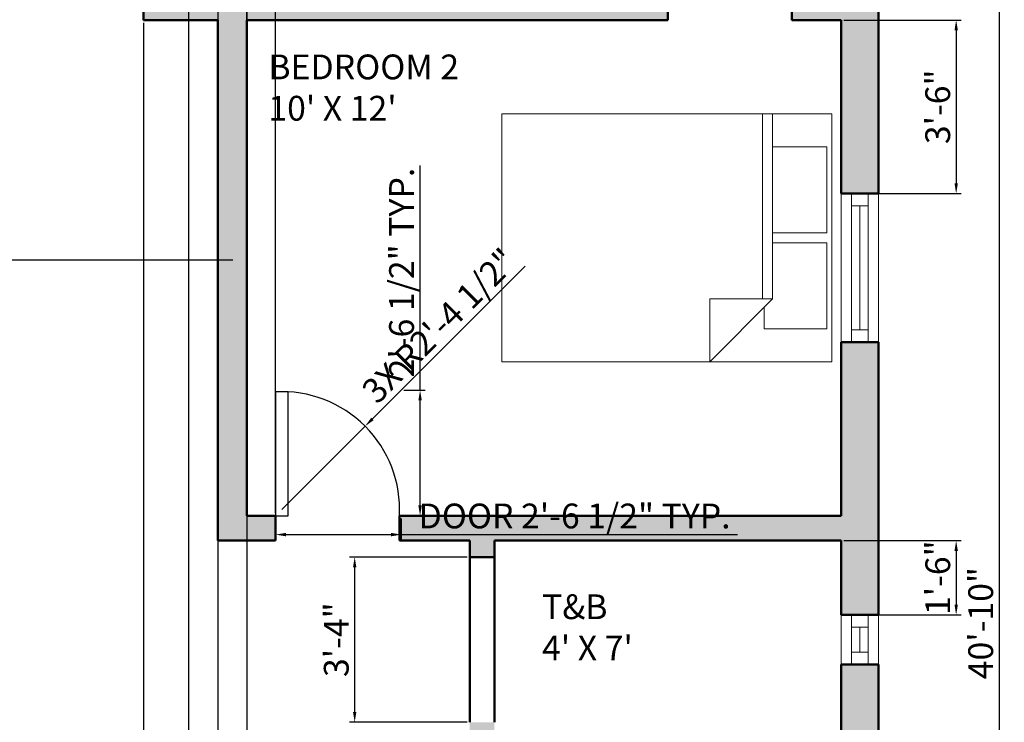
# Model space of a CAD drawing. Units: inches. Extents: x 2247 to 2697, y 1573 to 2133.
# Tile 3 of 4: x 2409 to 2648, y 1823 to 1993. Entities that reach past the tile are written whole.
import ezdxf

# ---------------------------------------------------------------- set-up
doc = ezdxf.new("R2010")
doc.units = ezdxf.units.IN
for name, color, linetype, lineweight in [('A-ANNO-DIMS', 2, 'Continuous', 18), ('A-AREA-IDEN', 7, 'Continuous', 25), ('A-DOOR', 4, 'Continuous', 25), ('A-FURN', 8, 'Continuous', 18), ('A-GLAZ', 4, 'Continuous', 18), ('A-WALL', 7, 'Continuous', 50)]:
    doc.layers.add(name, color=color, linetype=linetype, lineweight=lineweight)
doc.layers.add('A-WALL-PATT', color=67, linetype='Continuous', lineweight=13, true_color=0x727430)
doc.styles.get("Standard").update_dxf_attribs({"font": 'arial.ttf'})
doc.dimstyles.new('ISO-25', dxfattribs={"dimtxt": 6, "dimasz": 2.5, "dimexe": 1.25, "dimexo": 0.625, "dimtad": 1, "dimlunit": 3, "dimtxsty": 'Standard', "dimcen": 2.5, "dimadec": 0, "dimazin": 0, "dimtfac": 1, "dimtmove": 0, "dimatfit": 3, "dimfxl": 1, "dimarcsym": 0})

# ---------------------------------------------------------------- blocks, each defined once
blk = doc.blocks.new('*D2')
at = {"layer": 'A-ANNO-DIMS', "color": 0, "lineweight": -2, "transparency": 16777216}
for p, q in [((2617.72, 2092.36), (2647.6, 2092.36)), ((2646.35, 2089.86), (2646.35, 1604.86)), ((2617.72, 1602.36), (2647.6, 1602.36))]:
    blk.add_line(p, q, dxfattribs=at)
at = {"layer": 'A-ANNO-DIMS', "color": 0, "transparency": 16777216}
for points in [[(2645.94, 2089.86), (2646.77, 2089.86), (2646.35, 2092.36)], [(2645.94, 1604.86), (2646.77, 1604.86), (2646.35, 1602.36)]]:
    blk.add_solid(points, dxfattribs=at)
at = {"layer": 'Defpoints', "color": 0, "transparency": 16777216}
for p in [(2617.09, 2092.36), (2617.09, 1602.36), (2646.35, 1602.36)]:
    blk.add_point(p, dxfattribs=at)
at = {"layer": 'A-ANNO-DIMS', "color": 0, "transparency": 16777216, "insert": (2642.66, 1847.36), "char_height": 6, "attachment_point": 5, "rotation": 90}
blk.add_mtext('40\'-10"', dxfattribs=at)
blk = doc.blocks.new('Bed - Queen')
for p, q in [((0, -80.00003), (0, 0)), ((0, 0), (59.99999, 0)), ((59.99999, 0), (59.99999, -80.00003)), ((7.99999, -1.2), (28.79998, -1.2)), ((7.99999, -14.4), (7.99999, -1.2)), ((28.79998, -1.2), (28.79998, -14.4)), ((31.19999, -1.2), (51.99999, -1.2)), ((31.19999, -14.4), (31.19999, -1.2)), ((51.99999, -1.2), (51.99999, -16.4)), ((0, -14.4), (44.8, -14.4)), ((59.99999, -29.6), (44.8, -14.4)), ((44.8, -14.4), (44.8, -29.6)), ((51.99999, -16.4), (46.79936, -16.4)), ((44.8, -16.8), (0, -16.8)), ((44.8, -29.6), (59.99999, -29.6)), ((59.99999, -80.00003), (0, -80.00003))]:
    blk.add_line(p, q)
blk = doc.blocks.new('DOOR-SWING-30IN')
blk.add_lwpolyline([(0, 0), (3, 0), (3, 30), (0, 30)], close=True)
blk.add_arc((1.5, 1.5), 28.54, 356.9872, 93.0128)
blk = doc.blocks.new('WIN-36IN')
for p, q in [((0, 9), (36, 9)), ((0, 6.5), (36, 6.5)), ((3, 2.5), (3, 6.5)), ((33, 2.5), (33, 6.5)), ((0, 2.5), (36, 2.5)), ((3, 4.5), (33, 4.5)), ((0, 0), (36, 0))]:
    blk.add_line(p, q)
blk = doc.blocks.new('WIN-SASH-12IN')
for p, q in [((0, 0), (0, 12)), ((4, 0), (4, 12)), ((0, 9), (4, 9)), ((2, 3), (2, 9)), ((0, 3), (4, 3))]:
    blk.add_line(p, q)
blk = doc.blocks.new('*D11')
at = {"layer": 'A-ANNO-DIMS', "color": 0, "lineweight": -2, "transparency": 16777216}
for p, q in [((2471.09, 1872.73), (2471.09, 1867.55)), ((2501.52, 1872.73), (2501.52, 1867.55)), ((2473.59, 1868.8), (2499.02, 1868.8)), ((2501.52, 1868.8), (2583, 1868.8))]:
    blk.add_line(p, q, dxfattribs=at)
at = {"layer": 'A-ANNO-DIMS', "color": 0, "transparency": 16777216}
for points in [[(2473.59, 1869.21), (2473.59, 1868.38), (2471.09, 1868.8)], [(2499.02, 1869.21), (2499.02, 1868.38), (2501.52, 1868.8)]]:
    blk.add_solid(points, dxfattribs=at)
at = {"layer": 'Defpoints', "color": 0, "transparency": 16777216}
for p in [(2471.09, 1873.36), (2501.52, 1873.36), (2501.52, 1868.8)]:
    blk.add_point(p, dxfattribs=at)
at = {"layer": 'A-ANNO-DIMS', "color": 0, "transparency": 16777216, "insert": (2543.51, 1872.53), "char_height": 6, "attachment_point": 5}
blk.add_mtext('DOOR 2\'-6 1/2" TYP.', dxfattribs=at)
blk = doc.blocks.new('*D12')
at = {"layer": 'A-ANNO-DIMS', "color": 0, "lineweight": -2, "transparency": 16777216}
for p, q in [((2506.08, 1903.78), (2506.08, 1958.19)), ((2502.14, 1903.78), (2507.33, 1903.78)), ((2506.08, 1875.86), (2506.08, 1901.28)), ((2502.14, 1873.36), (2507.33, 1873.36))]:
    blk.add_line(p, q, dxfattribs=at)
at = {"layer": 'A-ANNO-DIMS', "color": 0, "transparency": 16777216}
for points in [[(2505.67, 1901.28), (2506.5, 1901.28), (2506.08, 1903.78)], [(2505.67, 1875.86), (2506.5, 1875.86), (2506.08, 1873.36)]]:
    blk.add_solid(points, dxfattribs=at)
at = {"layer": 'Defpoints', "color": 0, "transparency": 16777216}
for p in [(2501.52, 1903.78), (2506.08, 1903.78), (2501.52, 1873.36)]:
    blk.add_point(p, dxfattribs=at)
at = {"layer": 'A-ANNO-DIMS', "color": 0, "transparency": 16777216, "insert": (2502.36, 1932.24), "char_height": 6, "attachment_point": 5, "rotation": 90}
blk.add_mtext('2\'-6 1/2" TYP.', dxfattribs=at)
blk = doc.blocks.new('*D26')
at = {"layer": 'A-ANNO-DIMS', "color": 0, "lineweight": -2, "transparency": 16777216}
for p, q in [((2457.09, 2052.73), (2457.09, 1573.26)), ((2464.09, 2052.73), (2464.09, 1573.26)), ((2459.59, 1574.51), (2461.59, 1574.51)), ((2464.09, 1574.51), (2483.79, 1574.51))]:
    blk.add_line(p, q, dxfattribs=at)
at = {"layer": 'A-ANNO-DIMS', "color": 0, "transparency": 16777216}
for points in [[(2459.59, 1574.93), (2459.59, 1574.09), (2457.09, 1574.51)], [(2461.59, 1574.93), (2461.59, 1574.09), (2464.09, 1574.51)]]:
    blk.add_solid(points, dxfattribs=at)
at = {"layer": 'Defpoints', "color": 0, "transparency": 16777216}
for p in [(2457.09, 2053.36), (2464.09, 2053.36), (2464.09, 1574.51)]:
    blk.add_point(p, dxfattribs=at)
at = {"layer": 'A-ANNO-DIMS', "color": 0, "transparency": 16777216, "insert": (2475.19, 1578.2), "char_height": 6, "attachment_point": 5}
blk.add_mtext('0\'-7"', dxfattribs=at)
blk = doc.blocks.new('*D28')
at = {"layer": 'A-ANNO-DIMS', "color": 0, "lineweight": -2, "transparency": 16777216}
for p, q in [((2608.72, 1993.36), (2637.19, 1993.36)), ((2635.94, 1990.86), (2635.94, 1953.86)), ((2608.72, 1951.36), (2637.19, 1951.36))]:
    blk.add_line(p, q, dxfattribs=at)
at = {"layer": 'A-ANNO-DIMS', "color": 0, "transparency": 16777216}
for points in [[(2635.53, 1990.86), (2636.36, 1990.86), (2635.94, 1993.36)], [(2635.53, 1953.86), (2636.36, 1953.86), (2635.94, 1951.36)]]:
    blk.add_solid(points, dxfattribs=at)
at = {"layer": 'Defpoints', "color": 0, "transparency": 16777216}
for p in [(2608.09, 1993.36), (2608.09, 1951.36), (2635.94, 1951.36)]:
    blk.add_point(p, dxfattribs=at)
at = {"layer": 'A-ANNO-DIMS', "color": 0, "transparency": 16777216, "insert": (2632.25, 1972.36), "char_height": 6, "attachment_point": 5, "rotation": 90}
blk.add_mtext('3\'-6"', dxfattribs=at)
blk = doc.blocks.new('*D29')
at = {"layer": 'A-ANNO-DIMS', "color": 0, "lineweight": -2, "transparency": 16777216}
for p, q in [((2608.72, 1867.36), (2637.19, 1867.36)), ((2635.94, 1864.86), (2635.94, 1851.86)), ((2608.72, 1849.36), (2637.19, 1849.36))]:
    blk.add_line(p, q, dxfattribs=at)
at = {"layer": 'A-ANNO-DIMS', "color": 0, "transparency": 16777216}
for points in [[(2635.53, 1864.86), (2636.36, 1864.86), (2635.94, 1867.36)], [(2635.53, 1851.86), (2636.36, 1851.86), (2635.94, 1849.36)]]:
    blk.add_solid(points, dxfattribs=at)
at = {"layer": 'Defpoints', "color": 0, "transparency": 16777216}
for p in [(2608.09, 1867.36), (2608.09, 1849.36), (2635.94, 1849.36)]:
    blk.add_point(p, dxfattribs=at)
at = {"layer": 'A-ANNO-DIMS', "color": 0, "transparency": 16777216, "insert": (2632.26, 1858.36), "char_height": 6, "attachment_point": 5, "rotation": 90}
blk.add_mtext('1\'-6"', dxfattribs=at)
blk = doc.blocks.new('*D38')
at = {"layer": 'A-ANNO-DIMS', "color": 0, "lineweight": -2, "transparency": 16777216}
for p, q in [((2390.09, 1693.98), (2390.09, 2121.46)), ((2450.09, 1693.98), (2450.09, 2121.46)), ((2392.59, 2120.21), (2447.59, 2120.21))]:
    blk.add_line(p, q, dxfattribs=at)
at = {"layer": 'A-ANNO-DIMS', "color": 0, "transparency": 16777216}
for points in [[(2392.59, 2120.63), (2392.59, 2119.79), (2390.09, 2120.21)], [(2447.59, 2120.63), (2447.59, 2119.79), (2450.09, 2120.21)]]:
    blk.add_solid(points, dxfattribs=at)
at = {"layer": 'Defpoints', "color": 0, "transparency": 16777216}
for p in [(2450.09, 2120.21), (2390.09, 1693.36), (2450.09, 1693.36)]:
    blk.add_point(p, dxfattribs=at)
at = {"layer": 'A-ANNO-DIMS', "color": 0, "transparency": 16777216, "insert": (2420.09, 2123.9), "char_height": 6, "attachment_point": 5}
blk.add_mtext('5\'-0"', dxfattribs=at)
blk = doc.blocks.new('*D40')
at = {"layer": 'A-ANNO-DIMS', "color": 0, "lineweight": -2, "transparency": 16777216}
for p, q in [((2391.09, 1992.73), (2391.09, 1573.26)), ((2439.09, 1992.73), (2439.09, 1573.26)), ((2393.59, 1574.51), (2436.59, 1574.51))]:
    blk.add_line(p, q, dxfattribs=at)
at = {"layer": 'A-ANNO-DIMS', "color": 0, "transparency": 16777216}
for points in [[(2393.59, 1574.93), (2393.59, 1574.09), (2391.09, 1574.51)], [(2436.59, 1574.93), (2436.59, 1574.09), (2439.09, 1574.51)]]:
    blk.add_solid(points, dxfattribs=at)
at = {"layer": 'Defpoints', "color": 0, "transparency": 16777216}
for p in [(2391.09, 1993.36), (2439.09, 1993.36), (2439.09, 1574.51)]:
    blk.add_point(p, dxfattribs=at)
at = {"layer": 'A-ANNO-DIMS', "color": 0, "transparency": 16777216, "insert": (2415.09, 1578.2), "char_height": 6, "attachment_point": 5}
blk.add_mtext('4\'-0"', dxfattribs=at)
blk = doc.blocks.new('*D42')
at = {"layer": 'A-ANNO-DIMS', "color": 0, "lineweight": -2, "transparency": 16777216}
for p, q in [((2464.09, 1873.98), (2464.09, 2121.46)), ((2471.09, 1873.98), (2471.09, 2121.46)), ((2466.59, 2120.21), (2468.59, 2120.21)), ((2471.09, 2120.21), (2490.79, 2120.21))]:
    blk.add_line(p, q, dxfattribs=at)
at = {"layer": 'A-ANNO-DIMS', "color": 0, "transparency": 16777216}
for points in [[(2466.59, 2120.63), (2466.59, 2119.79), (2464.09, 2120.21)], [(2468.59, 2120.63), (2468.59, 2119.79), (2471.09, 2120.21)]]:
    blk.add_solid(points, dxfattribs=at)
at = {"layer": 'Defpoints', "color": 0, "transparency": 16777216}
for p in [(2471.09, 2120.21), (2464.09, 1873.36), (2471.09, 1873.36)]:
    blk.add_point(p, dxfattribs=at)
at = {"layer": 'A-ANNO-DIMS', "color": 0, "transparency": 16777216, "insert": (2482.19, 2123.9), "char_height": 6, "attachment_point": 5}
blk.add_mtext('0\'-7"', dxfattribs=at)
blk = doc.blocks.new('*D44')
at = {"layer": 'A-ANNO-DIMS', "color": 0, "lineweight": -2, "transparency": 16777216}
for p, q in [((2517.47, 1863.36), (2488.99, 1863.36)), ((2490.24, 1825.86), (2490.24, 1860.86)), ((2517.47, 1823.36), (2488.99, 1823.36))]:
    blk.add_line(p, q, dxfattribs=at)
at = {"layer": 'A-ANNO-DIMS', "color": 0, "transparency": 16777216}
for points in [[(2489.83, 1860.86), (2490.66, 1860.86), (2490.24, 1863.36)], [(2489.83, 1825.86), (2490.66, 1825.86), (2490.24, 1823.36)]]:
    blk.add_solid(points, dxfattribs=at)
at = {"layer": 'Defpoints', "color": 0, "transparency": 16777216}
for p in [(2490.24, 1863.36), (2518.09, 1863.36), (2518.09, 1823.36)]:
    blk.add_point(p, dxfattribs=at)
at = {"layer": 'A-ANNO-DIMS', "color": 0, "transparency": 16777216, "insert": (2486.55, 1843.36), "char_height": 6, "attachment_point": 5, "rotation": 90}
blk.add_mtext('3\'-4"', dxfattribs=at)
blk = doc.blocks.new('*D49')
at = {"layer": 'A-ANNO-DIMS', "color": 0, "lineweight": -2, "transparency": 16777216}
for p, q in [((2252.99, 1935.2), (2337.01, 1935.2)), ((2460.71, 1935.2), (2339.51, 1935.2))]:
    blk.add_line(p, q, dxfattribs=at)
at = {"layer": 'A-ANNO-DIMS', "color": 0, "transparency": 16777216}
blk.add_solid([(2337.01, 1935.62), (2337.01, 1934.79), (2339.51, 1935.2)], dxfattribs=at)
at = {"layer": 'Defpoints', "color": 0, "transparency": 16777216}
for p in [(2339.51, 1935.2), (2460.71, 1935.2)]:
    blk.add_point(p, dxfattribs=at)
at = {"layer": 'A-ANNO-DIMS', "color": 0, "transparency": 16777216, "insert": (2266.79, 1938.89), "char_height": 6, "attachment_point": 5}
blk.add_mtext('R10\'-1"', dxfattribs=at)
blk = doc.blocks.new('*D50')
at = {"layer": 'A-ANNO-DIMS', "color": 0, "lineweight": -2, "transparency": 16777216}
for p, q in [((2246.5, 1935.2), (2331.01, 1935.2)), ((2447.76, 1935.2), (2333.51, 1935.2))]:
    blk.add_line(p, q, dxfattribs=at)
at = {"layer": 'A-ANNO-DIMS', "color": 0, "transparency": 16777216}
blk.add_solid([(2331.01, 1935.62), (2331.01, 1934.79), (2333.51, 1935.2)], dxfattribs=at)
at = {"layer": 'Defpoints', "color": 0, "transparency": 16777216}
for p in [(2333.51, 1935.2), (2447.76, 1935.2)]:
    blk.add_point(p, dxfattribs=at)
at = {"layer": 'A-ANNO-DIMS', "color": 0, "transparency": 16777216, "insert": (2264.96, 1938.93), "char_height": 6, "attachment_point": 5}
blk.add_mtext('R9\'-6 1/2"', dxfattribs=at)
blk = doc.blocks.new('*D51')
at = {"layer": 'A-ANNO-DIMS', "color": 0, "lineweight": -2, "transparency": 16777216}
for p, q in [((2531.53, 1933.8), (2494.54, 1896.81)), ((2472.59, 1874.86), (2492.77, 1895.04))]:
    blk.add_line(p, q, dxfattribs=at)
at = {"layer": 'A-ANNO-DIMS', "color": 0, "transparency": 16777216}
blk.add_solid([(2494.25, 1897.1), (2494.84, 1896.51), (2492.77, 1895.04)], dxfattribs=at)
at = {"layer": 'Defpoints', "color": 0, "transparency": 16777216}
for p in [(2492.77, 1895.04), (2472.59, 1874.86)]:
    blk.add_point(p, dxfattribs=at)
at = {"layer": 'A-ANNO-DIMS', "color": 0, "transparency": 16777216, "insert": (2511.28, 1918.82), "char_height": 6, "attachment_point": 5, "rotation": 44.9996}
blk.add_mtext('3X R2\'-4 1/2"', dxfattribs=at)

msp = doc.modelspace()

# ---------------------------------------------------------------- hatches: boundary and pattern name
at = {"layer": 'A-WALL-PATT'}
h = msp.add_hatch(color=256, dxfattribs=at)
h.dxf.hatch_style = 1
h.paths.add_polyline_path([(2566.094, 1999.36), (2559.094, 1999.36), (2559.094, 2083.36), (2607.094, 2083.36), (2607.094, 2047.36), (2617.094, 2047.36), (2617.094, 2092.36), (2526.594, 2092.36), (2526.594, 2083.36), (2553.094, 2083.36), (2553.094, 1999.36), (2464.094, 1999.36), (2439.094, 1999.36), (2439.094, 1993.36), (2457.094, 1993.36), (2457.094, 1867.36), (2471.094, 1867.36), (2471.094, 1873.36), (2464.094, 1873.36), (2464.094, 1993.36), (2566.094, 1993.36)])
h = msp.add_hatch(color=256, dxfattribs=at)
h.dxf.hatch_style = 1
h.paths.add_polyline_path([(2617.094, 2035.36), (2607.094, 2035.36), (2607.094, 1999.36), (2596.094, 1999.36), (2596.094, 1993.36), (2608.094, 1993.36), (2608.094, 1951.36), (2617.094, 1951.36)])
h = msp.add_hatch(color=256, dxfattribs=at)
h.dxf.hatch_style = 1
h.paths.add_polyline_path([(2617.094, 1915.36), (2608.094, 1915.36), (2608.094, 1873.36), (2501.094, 1873.36), (2501.094, 1867.36), (2518.094, 1867.36), (2518.094, 1863.36), (2524.094, 1863.36), (2524.094, 1867.36), (2608.094, 1867.36), (2608.094, 1849.36), (2617.094, 1849.36)])
h = msp.add_hatch(color=256, dxfattribs=at)
h.dxf.hatch_style = 1
h.paths.add_polyline_path([(2617.094, 1837.36), (2608.094, 1837.36), (2608.094, 1819.36), (2524.094, 1819.36), (2524.094, 1823.36), (2518.094, 1823.36), (2518.094, 1819.36), (2501.094, 1819.36), (2501.094, 1813.36), (2608.094, 1813.36), (2608.094, 1771.36), (2617.094, 1771.36)])

# ---------------------------------------------------------------- linework, layer by layer
at = {"layer": 'A-GLAZ'}
for p, q in [((2608.094, 1849.36), (2608.094, 1837.36)), ((2617.094, 1837.36), (2617.094, 1849.36))]:
    msp.add_line(p, q, dxfattribs=at)
at = {"layer": 'A-WALL'}
for p, q in [((2439.094, 1993.36), (2439.094, 1999.36)), ((2566.094, 1999.36), (2566.094, 1993.36)), ((2596.094, 1999.36), (2596.094, 1993.36)), ((2439.094, 1993.36), (2457.094, 1993.36)), ((2457.094, 1867.36), (2457.094, 1993.36)), ((2464.094, 1993.36), (2464.094, 1873.36)), ((2464.094, 1993.36), (2566.094, 1993.36)), ((2596.094, 1993.36), (2608.094, 1993.36)), ((2608.094, 1993.36), (2608.094, 1951.36)), ((2608.094, 1951.36), (2617.094, 1951.36)), ((2608.094, 1915.36), (2617.094, 1915.36)), ((2608.094, 1915.36), (2608.094, 1873.36)), ((2464.094, 1873.36), (2471.094, 1873.36)), ((2471.094, 1873.36), (2471.094, 1867.36)), ((2501.094, 1873.36), (2501.094, 1867.36)), ((2501.094, 1873.36), (2608.094, 1873.36)), ((2457.094, 1867.36), (2471.094, 1867.36)), ((2501.094, 1867.36), (2518.094, 1867.36)), ((2518.094, 1867.36), (2518.094, 1863.36)), ((2524.094, 1867.36), (2524.094, 1863.36)), ((2524.094, 1867.36), (2608.094, 1867.36)), ((2608.094, 1867.36), (2608.094, 1849.36)), ((2518.094, 1863.36), (2524.094, 1863.36)), ((2518.094, 1823.36), (2518.094, 1863.36)), ((2524.094, 1823.36), (2524.094, 1863.36)), ((2608.094, 1849.36), (2617.094, 1849.36)), ((2608.094, 1837.36), (2617.094, 1837.36)), ((2608.094, 1837.36), (2608.094, 1819.36))]:
    msp.add_line(p, q, dxfattribs=at)
for points in [[(2617.094, 2035.36), (2617.094, 1951.36)], [(2617.094, 1915.36), (2617.094, 1849.36)], [(2617.094, 1837.36), (2617.094, 1771.36)]]:
    msp.add_lwpolyline(points, dxfattribs=at)

# ---------------------------------------------------------------- block references
at = {"layer": 'A-DOOR'}
msp.add_blockref('DOOR-SWING-30IN', (2471.094, 1873.36), dxfattribs=at)
at = {"layer": 'A-FURN', "rotation": 270}
msp.add_blockref('Bed - Queen', (2605.851, 1970.648), dxfattribs=at)
at = {"layer": 'A-GLAZ'}
for name, p, rotation in [('WIN-36IN', (2608.095, 1951.36), 270.0000000000049), ('WIN-SASH-12IN', (2614.595, 1849.359), 180)]:
    msp.add_blockref(name, p, dxfattribs=dict(at, rotation=rotation))

# ---------------------------------------------------------------- texts
at = {"layer": 'A-AREA-IDEN', "char_height": 6, "attachment_point": 1}
for s, width, insert in [("{\\fArial|b1|i0|c0|p34;BEDROOM 2 \\P10' X 12'}", 104.07009, (2469.331, 1985.018)), ("{\\fArial|b1|i0|c0|p34;T&B \\P4' X 7'}", 43.11494, (2535.625, 1854.335))]:
    msp.add_mtext_dynamic_manual_height_columns(s, width=width, gutter_width=12.5, heights=[0], dxfattribs=dict(at, insert=insert))

# ---------------------------------------------------------------- dimensions: what is measured, and where the dimension line sits
at = {"layer": 'A-ANNO-DIMS'}
for base, p1, p2, picture, middle in [((2450.094, 2120.21), (2390.094, 1693.36), (2450.094, 1693.36), '*D38', (2420.094, 2123.898)), ((2471.094, 2120.21), (2464.094, 1873.36), (2471.094, 1873.36), '*D42', (2482.194, 2123.898)), ((2464.094, 1574.51), (2457.094, 2053.36), (2464.094, 2053.36), '*D26', (2475.194, 1578.198)), ((2439.094, 1574.51), (2391.094, 1993.36), (2439.094, 1993.36), '*D40', (2415.094, 1578.198))]:
    dim = msp.add_linear_dim(base=base, p1=p1, p2=p2, dimstyle='ISO-25', override={"dimdec": 1, "dimlfac": 1, "dimrnd": 0, "dimzin": 1, "dimdsep": 46, "dimlunit": 4, "dimfrac": 2}, dxfattribs=at)
    dim.commit()
    dim.dimension.update_dxf_attribs({"geometry": picture, "text_midpoint": middle})
for base, p1, p2, angle, override, picture, middle in [((2646.352, 1602.36), (2617.094, 2092.36), (2617.094, 1602.36), 90, {"dimclrd": 0, "dimclre": 0, "dimclrt": 0}, '*D2', (2642.664, 1847.36)), ((2635.944, 1951.36), (2608.094, 1993.36), (2608.094, 1951.36), 270, {"dimdec": 1, "dimlfac": 1, "dimrnd": 0, "dimzin": 1, "dimdsep": 46, "dimlunit": 4, "dimfrac": 2}, '*D28', (2632.254, 1972.36)), ((2635.944, 1849.36), (2608.094, 1867.36), (2608.094, 1849.36), 270, {"dimdec": 1, "dimlfac": 1, "dimrnd": 0, "dimzin": 1, "dimdsep": 46, "dimlunit": 4, "dimfrac": 2}, '*D29', (2632.256, 1858.36)), ((2490.244, 1863.36), (2518.094, 1823.36), (2518.094, 1863.36), 90, {"dimdec": 1, "dimlfac": 1, "dimrnd": 0, "dimzin": 1, "dimdsep": 46, "dimlunit": 4, "dimfrac": 2}, '*D44', (2486.554, 1843.36))]:
    dim = msp.add_linear_dim(base=base, p1=p1, p2=p2, angle=angle, dimstyle='ISO-25', override=override, dxfattribs=at)
    dim.commit()
    dim.dimension.update_dxf_attribs({"geometry": picture, "text_midpoint": middle})
dim = msp.add_linear_dim(base=(2506.083, 1903.785), p1=(2501.52, 1873.36), p2=(2501.52, 1903.785), angle=90, text='<> TYP.', dimstyle='ISO-25', override={"dimdec": 1, "dimlfac": 1, "dimrnd": 0, "dimzin": 1, "dimdsep": 46, "dimlunit": 4, "dimfrac": 2}, dxfattribs=at)
dim.commit()
dim.dimension.update_dxf_attribs({"geometry": '*D12', "text_midpoint": (2502.356, 1932.238)})
for center, mpoint, picture, middle in [((2447.762936, 1935.202052), (2333.512936, 1935.202), '*D50', (2264.962936, 1935.202)), ((2460.71, 1935.202), (2339.513, 1935.202), '*D49', (2266.795, 1935.202))]:
    dim = msp.add_radius_dim(center=center, mpoint=mpoint, dimstyle='ISO-25', override={"dimdec": 1, "dimlfac": 1, "dimrnd": 0, "dimzin": 1, "dimdsep": 46, "dimlunit": 4, "dimfrac": 2}, dxfattribs=at)
    dim.commit()
    dim.dimension.update_dxf_attribs({"geometry": picture, "text_midpoint": middle, "dimtype": 164})
dim = msp.add_radius_dim(center=(2472.594, 1874.86), mpoint=(2492.775, 1895.04), text='3X <>', dimstyle='ISO-25', override={"dimdec": 1, "dimlfac": 1, "dimrnd": 0, "dimzin": 1, "dimdsep": 46, "dimlunit": 4, "dimfrac": 2}, dxfattribs=at)
dim.commit()
dim.dimension.update_dxf_attribs({"geometry": '*D51', "text_midpoint": (2511.284, 1918.823)})
dim = msp.add_linear_dim(base=(2501.52, 1868.796), p1=(2471.094, 1873.36), p2=(2501.52, 1873.36), text='DOOR <> TYP.', dimstyle='ISO-25', override={"dimdec": 1, "dimlfac": 1, "dimrnd": 0, "dimzin": 1, "dimdsep": 46, "dimlunit": 4, "dimfrac": 2}, dxfattribs=at)
dim.commit()
dim.dimension.update_dxf_attribs({"geometry": '*D11', "text_midpoint": (2543.509, 1872.525)})

doc.saveas('drawing.dxf')
